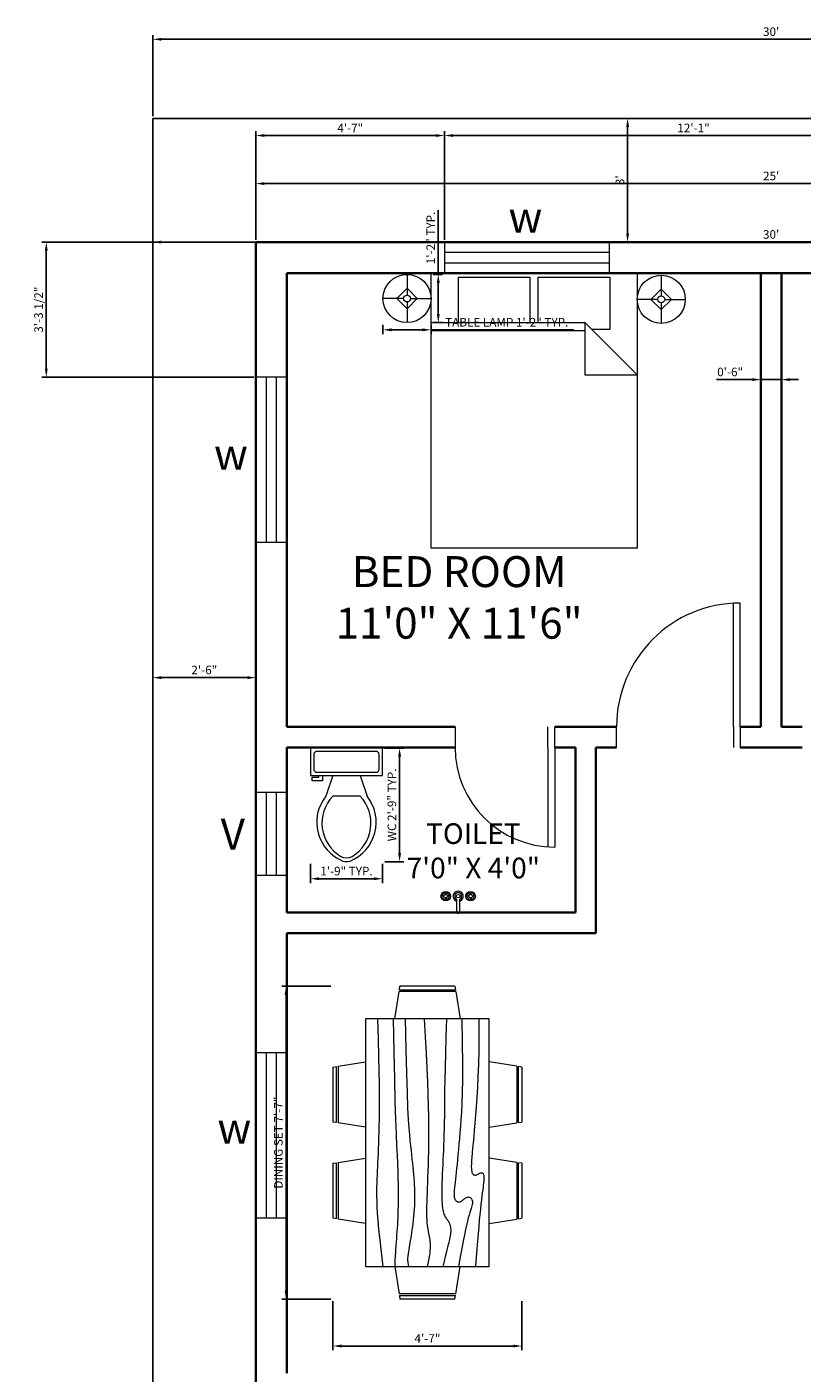
# Model space of a CAD drawing. Units: inches. Extents: x 2009 to 2890, y 2827 to 3504.
# Tile 2 of 6: x 2009 to 2235, y 3105 to 3496. Entities that reach past the tile are written whole.
import ezdxf

# ---------------------------------------------------------------- set-up
doc = ezdxf.new("R2010")
doc.units = ezdxf.units.IN
for name, color, linetype, lineweight in [('A-ANNO-DIMS', 2, 'Continuous', 18), ('A-ANNO-TEXT', 3, 'Continuous', 18), ('A-AREA-IDEN', 7, 'Continuous', 25), ('A-DOOR', 3, 'Continuous', 18), ('A-FLOR-FIXT', 9, 'Continuous', 18), ('A-FURN', 8, 'Continuous', 18), ('A-GLAZ', 4, 'Continuous', 18), ('A-WALL', 7, 'Continuous', 35), ('C-PROP', 8, 'Continuous', 25)]:
    doc.layers.add(name, color=color, linetype=linetype, lineweight=lineweight)
doc.styles.get("Standard").update_dxf_attribs({"font": 'arial.ttf'})
doc.dimstyles.new('ISO-25', dxfattribs={"dimtxt": 2.5, "dimasz": 2.5, "dimexe": 1.25, "dimexo": 0.625, "dimtad": 1, "dimdec": 0, "dimlunit": 3, "dimtxsty": 'Standard', "dimcen": 2.5, "dimadec": 0, "dimazin": 0, "dimtfac": 1, "dimtdec": 0, "dimtmove": 0, "dimatfit": 3, "dimfxl": 1, "dimarcsym": 0})

# ---------------------------------------------------------------- blocks, each defined once
blk = doc.blocks.new('Dining Set - 36 x 72 in.')
for p, q in [((-22, 27.5), (-22.1562, 26.50042)), ((-22, 27.5), (-6, 27.5)), ((-5.8437, 26.49966), (-6, 27.5)), ((6, 27.5), (5.8438, 26.50042)), ((6, 27.5), (22, 27.5)), ((22.1563, 26.49966), (22, 27.5)), ((-22.2343, 26.00059), (-23.4847, 17.99762)), ((-22.2304, 26), (-5.7608, 26)), ((-5.8416, 26.5), (-22.1534, 26.5)), ((-4.5152, 17.99762), (-5.7655, 25.99926)), ((5.7657, 26.00059), (4.5153, 17.99762)), ((5.7696, 26), (22.2392, 26)), ((22.1584, 26.5), (5.8466, 26.5)), ((23.4848, 17.99762), (22.2345, 25.99926)), ((36, 18), (-36, 18)), ((-36, 18), (-36, -18)), ((36, -18), (36, 18)), ((-45.5, 8), (-44.5004, 8.15617)), ((-45.5, 8), (-45.5, -8)), ((-44.5, -8.15843), (-44.5, 8.15338)), ((-44.0006, 8.23428), (-35.9976, 9.48474)), ((-44, 8.23041), (-44, -8.23915)), ((44.0006, 8.23428), (35.9976, 9.48474)), ((44, 8.23041), (44, -8.23915)), ((44.5, -8.15843), (44.5, 8.15338)), ((45.5, 8), (44.5005, 8.15617)), ((45.5, 8), (45.5, -8)), ((-44.4997, -8.15631), (-45.5, -8)), ((-35.9976, -9.48476), (-43.9993, -8.2345)), ((35.9976, -9.48476), (43.9993, -8.2345)), ((44.4997, -8.15631), (45.5, -8)), ((-36, -18), (36, -18)), ((-22.2343, -26.0006), (-23.4847, -17.99762)), ((-4.5152, -17.99762), (-5.7655, -25.99928)), ((5.7657, -26.0006), (4.5153, -17.99762)), ((23.4848, -17.99762), (22.2345, -25.99928)), ((-22.2304, -26), (-5.7608, -26)), ((-22, -27.5), (-22.1562, -26.50044)), ((-5.8416, -26.5), (-22.1534, -26.5)), ((-5.8437, -26.49967), (-6, -27.5)), ((5.7696, -26), (22.2392, -26)), ((6, -27.5), (5.8438, -26.50044)), ((22.1584, -26.5), (5.8466, -26.5)), ((22.1563, -26.49967), (22, -27.5)), ((-22, -27.5), (-6, -27.5)), ((6, -27.5), (22, -27.5))]:
    blk.add_line(p, q)
for points in [[(-36, 15), (-31.1772, 14.97754), (-26.8079, 14.91406), (-22.8538, 14.81543), (-19.276, 14.6875), (-16.0362, 14.53613), (-13.0957, 14.36718), (-10.4159, 14.18652), (-7.9583, 14), (-5.6904, 13.81315), (-3.6035, 13.63021), (-1.6954, 13.45508), (0.0365, 13.29166), (1.5945, 13.14388), (2.9811, 13.01562), (4.1988, 12.9108), (5.25, 12.83333), (6.1393, 12.78613), (6.8802, 12.76823), (7.4883, 12.77767), (7.9792, 12.8125), (8.3685, 12.87077), (8.6719, 12.95052), (8.9049, 13.0498), (9.0833, 13.16666), (9.2205, 13.29899), (9.3216, 13.44401), (9.3895, 13.59879), (9.4271, 13.76041), (9.4373, 13.92594), (9.4232, 14.09245), (9.3875, 14.257), (9.3333, 14.41666), (9.2638, 14.56917), (9.1836, 14.71484), (9.0975, 14.85465), (9.0104, 14.98958), (8.9272, 15.1206), (8.8529, 15.2487), (8.7922, 15.37483), (8.75, 15.5), (8.7305, 15.62467), (8.7344, 15.74739), (8.7617, 15.86621), (8.8125, 15.97916), (8.8867, 16.08431), (8.9844, 16.17968), (9.1055, 16.26334), (9.25, 16.33333), (9.4189, 16.38802), (9.6172, 16.42708), (9.8506, 16.45052), (10.125, 16.45833), (10.4463, 16.45052), (10.8203, 16.42708), (11.2529, 16.38802), (11.75, 16.33333), (12.3184, 16.26318), (12.9694, 16.17838), (13.7151, 16.07991), (14.5677, 15.96875), (15.5395, 15.84586), (16.6426, 15.71224), (17.8893, 15.56884), (19.2917, 15.41666), (20.859, 15.25667), (22.5879, 15.08984), (24.4721, 14.91715), (26.5052, 14.73958), (28.6809, 14.5581), (30.9929, 14.3737), (33.4347, 14.18733), (36, 14)], [(-36, 10), (-28.9766, 10.14274), (-23.1725, 10.20442), (-18.4241, 10.19775), (-14.5677, 10.13541), (-11.4399, 10.03011), (-8.877, 9.89453), (-6.7154, 9.74137), (-4.7917, 9.58333), (-2.9698, 9.43082), (-1.2246, 9.28515), (0.4415, 9.14534), (2.026, 9.01041), (3.5266, 8.87939), (4.9408, 8.7513), (6.266, 8.62516), (7.5, 8.5), (8.6411, 8.37549), (9.6914, 8.2539), (10.6538, 8.13818), (11.5312, 8.03125), (12.3267, 7.93603), (13.043, 7.85547), (13.6831, 7.79248), (14.25, 7.75), (14.7471, 7.7303), (15.1797, 7.73307), (15.5537, 7.75732), (15.875, 7.80208), (16.1494, 7.86637), (16.3828, 7.94922), (16.5811, 8.04964), (16.75, 8.16666), (16.8944, 8.29915), (17.0143, 8.44531), (17.1089, 8.60319), (17.1771, 8.77083), (17.218, 8.94629), (17.2305, 9.1276), (17.2137, 9.31282), (17.1667, 9.5), (17.0895, 9.6875), (16.987, 9.875), (16.8649, 10.0625), (16.7292, 10.25), (16.5856, 10.4375), (16.4401, 10.625), (16.2985, 10.8125), (16.1667, 11), (16.05, 11.18733), (15.9518, 11.3737), (15.8752, 11.5581), (15.8229, 11.73958), (15.798, 11.91715), (15.8034, 12.08984), (15.842, 12.25667), (15.9167, 12.41666), (16.0295, 12.56836), (16.1784, 12.70833), (16.3605, 12.83268), (16.5729, 12.9375), (16.8127, 13.01888), (17.0768, 13.07291), (17.3625, 13.0957), (17.6667, 13.08333), (17.9894, 13.03312), (18.3418, 12.94726), (18.7382, 12.82918), (19.1927, 12.68229), (19.7195, 12.51001), (20.3327, 12.31575), (21.0465, 12.10294), (21.875, 11.875), (22.8357, 11.63354), (23.959, 11.37304), (25.2786, 11.08618), (26.8282, 10.76562), (28.6414, 10.40405), (30.752, 9.99414), (33.1936, 9.52856), (36, 9)], [(-36, 5.5), (-30.7157, 5.3348), (-26.069, 5.20963), (-21.9946, 5.11767), (-18.4271, 5.05208), (-15.3009, 5.00602), (-12.5508, 4.97265), (-10.1112, 4.94515), (-7.9167, 4.91666), (-5.909, 4.88167), (-4.0586, 4.83984), (-2.3429, 4.79215), (-0.7396, 4.73958), (0.7739, 4.6831), (2.22, 4.6237), (3.6213, 4.56233), (5, 4.5), (6.373, 4.43782), (7.7344, 4.3776), (9.0723, 4.32129), (10.375, 4.27083), (11.6309, 4.22819), (12.8281, 4.19531), (13.9551, 4.17415), (15, 4.16666), (15.954, 4.17448), (16.819, 4.19791), (17.6001, 4.23698), (18.3021, 4.29166), (18.9299, 4.36198), (19.4883, 4.44791), (19.9823, 4.54948), (20.4167, 4.66666), (20.7969, 4.79899), (21.1302, 4.94401), (21.4245, 5.09879), (21.6875, 5.26041), (21.9271, 5.42594), (22.1511, 5.59245), (22.3672, 5.757), (22.5834, 5.91666), (22.8065, 6.06868), (23.0404, 6.21093), (23.2879, 6.34147), (23.5521, 6.45833), (23.8358, 6.55957), (24.142, 6.64323), (24.4735, 6.70735), (24.8334, 6.75), (25.2235, 6.76969), (25.642, 6.76692), (26.0858, 6.74267), (26.5521, 6.69791), (27.0379, 6.63362), (27.5404, 6.55078), (28.0565, 6.45036), (28.5834, 6.33333), (29.1242, 6.19987), (29.7071, 6.04687), (30.3661, 5.87044), (31.1354, 5.66666), (32.0493, 5.43164), (33.142, 5.16146), (34.4475, 4.85221), (36, 4.5)], [(-36, -1), (-30.7915, -0.6591), (-26.0195, -0.38216), (-21.6519, -0.16284), (-17.6563, 0.00521), (-14.0005, 0.12833), (-10.6523, 0.21289), (-7.5796, 0.26522), (-4.75, 0.29166), (-2.134, 0.29793), (0.2878, 0.28711), (2.5317, 0.26163), (4.6146, 0.22396), (6.5529, 0.17651), (8.3633, 0.12174), (10.0623, 0.06209), (11.6667, 0), (13.1899, -0.06201), (14.6341, -0.1211), (15.9982, -0.17432), (17.2813, -0.21875), (18.4823, -0.25147), (19.6003, -0.26953), (20.6343, -0.27002), (21.5834, -0.25), (22.4481, -0.20768), (23.2357, -0.14584), (23.9549, -0.06836), (24.6146, 0.02083), (25.2235, 0.11784), (25.7904, 0.21875), (26.3241, 0.31966), (26.8334, 0.41666), (27.3265, 0.50618), (27.8099, 0.58593), (28.2894, 0.65397), (28.7709, 0.70833), (29.2601, 0.74707), (29.763, 0.76823), (30.2855, 0.76985), (30.8334, 0.75), (31.4088, 0.70784), (31.9994, 0.64713), (32.589, 0.57275), (33.1615, 0.48958), (33.7008, 0.4025), (34.1908, 0.3164), (34.6153, 0.23616), (34.9584, 0.16666), (35.2099, 0.11165), (35.3848, 0.07031), (35.504, 0.04069), (35.5886, 0.02083), (35.6594, 0.00879), (35.7377, 0.0026), (35.8442, 0.00032), (36, 0)], [(-36, -6.5), (-27.1843, -6.31267), (-20.084, -6.1263), (-14.469, -5.9419), (-10.1094, -5.76042), (-6.7752, -5.58285), (-4.2363, -5.41016), (-2.2629, -5.24333), (-0.625, -5.08334), (0.8708, -4.93099), (2.2715, -4.78646), (3.5872, -4.64974), (4.8281, -4.52084), (6.0046, -4.39974), (7.127, -4.28646), (8.2053, -4.18099), (9.25, -4.08334), (10.2705, -3.99382), (11.2734, -3.91407), (12.2647, -3.84603), (13.25, -3.79167), (14.2354, -3.75293), (15.2266, -3.73177), (16.2295, -3.73015), (17.25, -3.75), (18.2912, -3.79248), (19.3451, -3.85547), (20.4009, -3.93604), (21.4479, -4.03125), (22.4754, -4.13819), (23.4727, -4.25391), (24.4289, -4.37549), (25.3334, -4.5), (26.1785, -4.62492), (26.9694, -4.74935), (27.7145, -4.87281), (28.4219, -4.99479), (29.1, -5.11483), (29.7572, -5.23242), (30.4016, -5.34709), (31.0417, -5.45834), (31.6837, -5.56437), (32.3262, -5.65821), (32.9658, -5.73153), (33.599, -5.77604), (34.2224, -5.78345), (34.8327, -5.74545), (35.4264, -5.65373), (36, -5.5)], [(-36, -10), (-26.4022, -9.81299), (-18.4675, -9.62891), (-11.9839, -9.45069), (-6.7396, -9.28125), (-2.5226, -9.12354), (0.8789, -8.98047), (3.6769, -8.85498), (6.0833, -8.75), (8.2767, -8.66765), (10.3021, -8.60677), (12.1712, -8.56543), (13.8958, -8.54167), (15.4876, -8.53353), (16.9583, -8.53907), (18.3197, -8.55632), (19.5834, -8.58334), (20.7616, -8.61841), (21.8685, -8.66081), (22.9188, -8.71004), (23.9271, -8.76563), (24.9081, -8.82707), (25.8763, -8.89388), (26.8465, -8.96558), (27.8334, -9.04167), (28.8474, -9.12118), (29.8828, -9.20117), (30.93, -9.27824), (31.9792, -9.34896), (33.0205, -9.40991), (34.0443, -9.45768), (35.0407, -9.48885), (36, -9.5)], [(-36, -14.5), (-30.0881, -14.33513), (-25.0332, -14.21224), (-20.7312, -14.12647), (-17.0781, -14.07292), (-13.97, -14.04671), (-11.3027, -14.04297), (-8.9724, -14.05681), (-6.875, -14.08334), (-4.9224, -14.11833), (-3.0905, -14.16016), (-1.3709, -14.20785), (0.2448, -14.26042), (1.7647, -14.3169), (3.1973, -14.3763), (4.5507, -14.43767), (5.8333, -14.5), (7.0554, -14.5621), (8.235, -14.62175), (9.3922, -14.67652), (10.5469, -14.72396), (11.7192, -14.76164), (12.929, -14.78711), (14.1965, -14.79794), (15.5417, -14.79167), (16.9933, -14.76424), (18.6152, -14.70508), (20.4804, -14.60197), (22.6615, -14.44271), (25.2312, -14.21509), (28.2624, -13.9069), (31.8277, -13.50594), (36, -13)]]:
    blk.add_lwpolyline(points)
blk = doc.blocks.new('Toilet - top')
for p, q in [((9.5, -6), (9.5, -2)), ((-10, -8.5), (-8, -8.5)), ((-10, -9.5), (-10, -8.5)), ((-7, -9.5), (-10, -9.5)), ((-8, -8.5), (-8, -8)), ((-7, -8), (-7, -9.5)), ((-4, -8), (-6, -14)), ((4, -8), (6, -14)), ((4, -14), (-4, -14))]:
    blk.add_line(p, q)
blk.add_lwpolyline([(10.5, -8), (10.5, 0), (-10.5, 0), (-10.5, -8)], close=True)
for points in [[(-9.5, -2), (-9.5, -6)], [(8.5, -1), (-8.5, -1)], [(-8.5, -7), (8.5, -7)]]:
    blk.add_lwpolyline(points)
for centre, radius, start, end in [((-8.62, -1.88), 0.884, 81.8699, 188.1301), ((8.62, -1.88), 0.884, 351.8699, 98.1301), ((-8.62, -6.12), 0.884, 171.8699, 278.1301), ((8.62, -6.12), 0.884, 261.8699, 8.1301), ((3.52, -21.58), 12.17, 141.4691, 247.9714), ((4.2, -21.82), 11.33, 136.3677, 238.9468), ((-3.52, -21.58), 12.17, 292.0284, 38.5307), ((-4.2, -21.82), 11.33, 301.053, 43.6321), ((0, -27.88), 4, 245.7318, 294.2682), ((0, -29), 4, 254.8605, 285.1395)]:
    blk.add_arc(centre, radius, start, end)
blk = doc.blocks.new('Bed - Queen')
for p, q in [((0, -80.00003), (0, 0)), ((0, 0), (59.99999, 0)), ((59.99999, 0), (59.99999, -80.00003)), ((7.99999, -1.2), (28.79998, -1.2)), ((7.99999, -14.4), (7.99999, -1.2)), ((28.79998, -1.2), (28.79998, -14.4)), ((31.19999, -1.2), (51.99999, -1.2)), ((31.19999, -14.4), (31.19999, -1.2)), ((51.99999, -1.2), (51.99999, -16.4)), ((0, -14.4), (44.8, -14.4)), ((59.99999, -29.6), (44.8, -14.4)), ((44.8, -14.4), (44.8, -29.6)), ((44.8, -16.8), (0, -16.8)), ((51.99999, -16.4), (46.79936, -16.4)), ((44.8, -29.6), (59.99999, -29.6)), ((59.99999, -80.00003), (0, -80.00003))]:
    blk.add_line(p, q)
blk = doc.blocks.new('Lamp - Table')
for p, q in [((0, 7), (0, 1)), ((-1, 0), (-7, 0)), ((0, 3), (-3, 0)), ((-3, 0), (0, -3)), ((3, 0), (0, 3)), ((0, -3), (3, 0)), ((1, 0), (7, 0)), ((0, -1), (0, -7))]:
    blk.add_line(p, q)
for radius in [7, 1]:
    blk.add_circle((0, 0), radius)
blk = doc.blocks.new('*D8')
at = {"layer": 'A-ANNO-DIMS', "color": 0, "lineweight": -2, "transparency": 16777216}
for p, q in [((2075.76, 3434.16), (2075.76, 3451.81)), ((2078.26, 3450.56), (2373.26, 3450.56)), ((2375.76, 3434.16), (2375.76, 3451.81))]:
    blk.add_line(p, q, dxfattribs=at)
at = {"layer": 'A-ANNO-DIMS', "color": 0, "transparency": 16777216}
for points in [[(2078.26, 3450.97), (2078.26, 3450.14), (2075.76, 3450.56)], [(2373.26, 3450.97), (2373.26, 3450.14), (2375.76, 3450.56)]]:
    blk.add_solid(points, dxfattribs=at)
at = {"layer": 'Defpoints', "color": 0, "transparency": 16777216}
for p in [(2375.76, 3450.56), (2075.76, 3433.54), (2375.76, 3433.54)]:
    blk.add_point(p, dxfattribs=at)
at = {"layer": 'A-ANNO-DIMS', "color": 0, "transparency": 16777216, "insert": (2225.76, 3452.46), "char_height": 2.5, "attachment_point": 5}
blk.add_mtext("25'", dxfattribs=at)
blk = doc.blocks.new('*D10')
at = {"layer": 'A-ANNO-DIMS', "color": 0, "lineweight": -2, "transparency": 16777216}
for p, q in [((2045.76, 3470.16), (2045.76, 3493.78)), ((2405.76, 3470.16), (2405.76, 3493.78)), ((2048.26, 3492.53), (2403.26, 3492.53))]:
    blk.add_line(p, q, dxfattribs=at)
at = {"layer": 'A-ANNO-DIMS', "color": 0, "transparency": 16777216}
for points in [[(2048.26, 3492.95), (2048.26, 3492.11), (2045.76, 3492.53)], [(2403.26, 3492.95), (2403.26, 3492.11), (2405.76, 3492.53)]]:
    blk.add_solid(points, dxfattribs=at)
at = {"layer": 'Defpoints', "color": 0, "transparency": 16777216}
for p in [(2405.76, 3492.53), (2045.76, 3469.54), (2405.76, 3469.54)]:
    blk.add_point(p, dxfattribs=at)
at = {"layer": 'A-ANNO-DIMS', "color": 0, "transparency": 16777216, "insert": (2225.76, 3494.43), "char_height": 2.5, "attachment_point": 5}
blk.add_mtext("30'", dxfattribs=at)
blk = doc.blocks.new('Faucet - Bathroom top')
for p, q in [((-4.107, 0.125), (-4.375, 0.125)), ((-3.75, 0.4788), (-3.75, 0.75)), ((-3.5, 0.482), (-3.5, 0.75)), ((-3.1461, 0.125), (-2.875, 0.125)), ((3.143, 0.125), (2.875, 0.125)), ((3.5, 0.4788), (3.5, 0.75)), ((3.75, 0.482), (3.75, 0.75)), ((4.1039, 0.125), (4.375, 0.125)), ((-4.1039, -0.125), (-4.375, -0.125)), ((-3.75, -0.4821), (-3.75, -0.75)), ((-3.5, -0.4789), (-3.5, -0.75)), ((-3.143, -0.125), (-2.875, -0.125)), ((-0.5, -0.8639), (-0.5, -4.5)), ((0.5, -4.5), (0.5, -0.8631)), ((3.1461, -0.125), (2.875, -0.125)), ((3.5, -0.4821), (3.5, -0.75)), ((3.75, -0.4789), (3.75, -0.75)), ((4.107, -0.125), (4.375, -0.125))]:
    blk.add_line(p, q)
for centre, radius in [((-3.625, 0), 1.375), ((-4.625, 0), 0.2795), ((-3.625, 0), 0.5), ((-3.625, 1), 0.2795), ((-2.625, 0), 0.2795), ((0, 0), 0.5), ((3.625, 0), 1.375), ((2.625, 0), 0.2795), ((3.625, 0), 0.5), ((3.625, 1), 0.2795), ((4.625, 0), 0.2795), ((-3.625, -1), 0.2795), ((3.625, -1), 0.2795)]:
    blk.add_circle(centre, radius)
for centre, radius, start, end in [((-3.625, 0), 1, 105.2407, 164.2093), ((-3.625, 0), 1, 16.44125, 74.07887), ((0, 0), 1.5, 289.6514, 250.3603), ((0, 0), 1, 300.3431, 239.7554), ((3.625, 0), 1, 106.12, 164.0884), ((3.625, 0), 1, 16.23422, 73.90469), ((-3.625, 0), 1, 196.2342, 253.9047), ((-3.625, 0), 1, 286.12, 344.0884), ((3.625, 0), 1, 196.4413, 254.0789), ((3.625, 0), 1, 285.2407, 344.2093), ((0, -4.5), 0.5, 180, 0)]:
    blk.add_arc(centre, radius, start, end)
blk = doc.blocks.new('*D15')
at = {"layer": 'A-ANNO-DIMS', "color": 0, "lineweight": -2, "transparency": 16777216}
for p, q in [((2184.59, 3469.54), (2185.22, 3469.54)), ((2183.97, 3436.04), (2183.97, 3467.04)), ((2184.59, 3433.54), (2185.22, 3433.54))]:
    blk.add_line(p, q, dxfattribs=at)
at = {"layer": 'A-ANNO-DIMS', "color": 0, "transparency": 16777216}
for points in [[(2183.55, 3467.04), (2184.39, 3467.04), (2183.97, 3469.54)], [(2183.55, 3436.04), (2184.39, 3436.04), (2183.97, 3433.54)]]:
    blk.add_solid(points, dxfattribs=at)
at = {"layer": 'Defpoints', "color": 0, "transparency": 16777216}
for p in [(2183.97, 3469.54), (2183.97, 3469.54), (2183.97, 3433.54)]:
    blk.add_point(p, dxfattribs=at)
at = {"layer": 'A-ANNO-DIMS', "color": 0, "transparency": 16777216, "insert": (2182.07, 3451.54), "char_height": 2.5, "attachment_point": 5, "rotation": 90}
blk.add_mtext("3'", dxfattribs=at)
blk = doc.blocks.new('*D16')
at = {"layer": 'A-ANNO-DIMS', "color": 0, "lineweight": -2, "transparency": 16777216}
for p, q in [((2045.76, 3468.91), (2045.76, 3432.29)), ((2405.76, 3468.91), (2405.76, 3432.29)), ((2403.26, 3433.54), (2048.26, 3433.54))]:
    blk.add_line(p, q, dxfattribs=at)
at = {"layer": 'A-ANNO-DIMS', "color": 0, "transparency": 16777216}
for points in [[(2048.26, 3433.96), (2048.26, 3433.12), (2045.76, 3433.54)], [(2403.26, 3433.96), (2403.26, 3433.12), (2405.76, 3433.54)]]:
    blk.add_solid(points, dxfattribs=at)
at = {"layer": 'Defpoints', "color": 0, "transparency": 16777216}
for p in [(2045.76, 3469.54), (2405.76, 3469.54), (2045.76, 3433.54)]:
    blk.add_point(p, dxfattribs=at)
at = {"layer": 'A-ANNO-DIMS', "color": 0, "transparency": 16777216, "insert": (2225.76, 3435.44), "char_height": 2.5, "attachment_point": 5}
blk.add_mtext("30'", dxfattribs=at)
blk = doc.blocks.new('*D21')
at = {"layer": 'A-ANNO-DIMS', "color": 0, "lineweight": -2, "transparency": 16777216}
for p, q in [((2045.76, 3305.32), (2045.76, 3308.09)), ((2073.26, 3306.84), (2048.26, 3306.84)), ((2075.76, 3305.32), (2075.76, 3308.09))]:
    blk.add_line(p, q, dxfattribs=at)
at = {"layer": 'A-ANNO-DIMS', "color": 0, "transparency": 16777216}
for points in [[(2048.26, 3307.25), (2048.26, 3306.42), (2045.76, 3306.84)], [(2073.26, 3307.25), (2073.26, 3306.42), (2075.76, 3306.84)]]:
    blk.add_solid(points, dxfattribs=at)
at = {"layer": 'Defpoints', "color": 0, "transparency": 16777216}
for p in [(2045.76, 3306.84), (2045.76, 3304.69), (2075.76, 3304.69)]:
    blk.add_point(p, dxfattribs=at)
at = {"layer": 'A-ANNO-DIMS', "color": 0, "transparency": 16777216, "insert": (2060.76, 3308.74), "char_height": 2.5, "attachment_point": 5}
blk.add_mtext('2\'-6"', dxfattribs=at)
blk = doc.blocks.new('WIN-48IN')
for p, q in [((0, 48), (0, 0)), ((9, 48), (0, 48)), ((3, 48), (3, 0)), ((6, 0), (6, 48)), ((9, 0), (9, 48)), ((0, 0), (9, 0))]:
    blk.add_line(p, q)
blk = doc.blocks.new('VENT-24IN')
for p, q in [((0, 24), (0, 0)), ((9, 24), (0, 24)), ((3, 24), (3, 0)), ((6, 0), (6, 24)), ((9, 0), (9, 24)), ((0, 0), (9, 0))]:
    blk.add_line(p, q)
blk = doc.blocks.new('DOOR-29IN')
for p, q in [((0, 35), (0, 29)), ((27, 29), (27, 35)), ((29, 29), (29, 35)), ((27, 29), (27, 0)), ((29, 29), (29, 0))]:
    blk.add_line(p, q)
blk.add_arc((29, 29), 29, 180, 270)
blk = doc.blocks.new('DOOR-36IN')
for p, q in [((34, 6), (34, 42)), ((36, 6), (36, 42)), ((0, 0), (0, 6)), ((34, 6), (34, 0)), ((36, 6), (36, 0))]:
    blk.add_line(p, q)
blk.add_arc((36, 6), 36, 90, 180)
blk = doc.blocks.new('*D45')
at = {"layer": 'A-ANNO-DIMS', "color": 0, "lineweight": -2, "transparency": 16777216}
for p, q in [((2112.76, 3409.49), (2112.76, 3406.77)), ((2115.26, 3408.02), (2124.26, 3408.02)), ((2126.76, 3409.49), (2126.76, 3406.77)), ((2126.76, 3408.02), (2168.33, 3408.02))]:
    blk.add_line(p, q, dxfattribs=at)
at = {"layer": 'A-ANNO-DIMS', "color": 0, "transparency": 16777216}
for points in [[(2115.26, 3408.43), (2115.26, 3407.6), (2112.76, 3408.02)], [(2124.26, 3408.43), (2124.26, 3407.6), (2126.76, 3408.02)]]:
    blk.add_solid(points, dxfattribs=at)
at = {"layer": 'Defpoints', "color": 0, "transparency": 16777216}
for p in [(2112.76, 3410.12), (2126.76, 3410.12), (2126.76, 3408.02)]:
    blk.add_point(p, dxfattribs=at)
at = {"layer": 'A-ANNO-DIMS', "color": 0, "transparency": 16777216, "insert": (2148.79, 3409.9), "char_height": 2.5, "attachment_point": 5}
blk.add_mtext('TABLE LAMP 1\'-2" TYP.', dxfattribs=at)
blk = doc.blocks.new('*D46')
at = {"layer": 'A-ANNO-DIMS', "color": 0, "lineweight": -2, "transparency": 16777216}
for p, q in [((2128.86, 3424.12), (2128.86, 3442.87)), ((2127.38, 3424.12), (2130.11, 3424.12)), ((2128.86, 3412.62), (2128.86, 3421.62)), ((2127.38, 3410.12), (2130.11, 3410.12))]:
    blk.add_line(p, q, dxfattribs=at)
at = {"layer": 'A-ANNO-DIMS', "color": 0, "transparency": 16777216}
for points in [[(2128.44, 3421.62), (2129.28, 3421.62), (2128.86, 3424.12)], [(2128.44, 3412.62), (2129.28, 3412.62), (2128.86, 3410.12)]]:
    blk.add_solid(points, dxfattribs=at)
at = {"layer": 'Defpoints', "color": 0, "transparency": 16777216}
for p in [(2126.76, 3424.12), (2128.86, 3424.12), (2126.76, 3410.12)]:
    blk.add_point(p, dxfattribs=at)
at = {"layer": 'A-ANNO-DIMS', "color": 0, "transparency": 16777216, "insert": (2126.98, 3434.74), "char_height": 2.5, "attachment_point": 5, "rotation": 90}
blk.add_mtext('1\'-2" TYP.', dxfattribs=at)
blk = doc.blocks.new('*D47')
at = {"layer": 'A-ANNO-DIMS', "color": 0, "lineweight": -2, "transparency": 16777216}
for p, q in [((2113.27, 3286.35), (2118.85, 3286.35)), ((2117.6, 3255.8), (2117.6, 3283.85)), ((2113.27, 3253.3), (2118.85, 3253.3))]:
    blk.add_line(p, q, dxfattribs=at)
at = {"layer": 'A-ANNO-DIMS', "color": 0, "transparency": 16777216}
for points in [[(2117.18, 3283.85), (2118.02, 3283.85), (2117.6, 3286.35)], [(2117.18, 3255.8), (2118.02, 3255.8), (2117.6, 3253.3)]]:
    blk.add_solid(points, dxfattribs=at)
at = {"layer": 'Defpoints', "color": 0, "transparency": 16777216}
for p in [(2112.64, 3286.35), (2117.6, 3286.35), (2112.64, 3253.3)]:
    blk.add_point(p, dxfattribs=at)
at = {"layer": 'A-ANNO-DIMS', "color": 0, "transparency": 16777216, "insert": (2115.68, 3269.82), "char_height": 2.5, "attachment_point": 5, "rotation": 90}
blk.add_mtext('WC 2\'-9" TYP.', dxfattribs=at)
blk = doc.blocks.new('*D48')
at = {"layer": 'A-ANNO-DIMS', "color": 0, "lineweight": -2, "transparency": 16777216}
for p, q in [((2091.64, 3252.67), (2091.64, 3247.09)), ((2112.64, 3252.67), (2112.64, 3247.09)), ((2094.14, 3248.34), (2110.14, 3248.34))]:
    blk.add_line(p, q, dxfattribs=at)
at = {"layer": 'A-ANNO-DIMS', "color": 0, "transparency": 16777216}
for points in [[(2094.14, 3248.76), (2094.14, 3247.93), (2091.64, 3248.34)], [(2110.14, 3248.76), (2110.14, 3247.93), (2112.64, 3248.34)]]:
    blk.add_solid(points, dxfattribs=at)
at = {"layer": 'Defpoints', "color": 0, "transparency": 16777216}
for p in [(2091.64, 3253.3), (2112.64, 3253.3), (2112.64, 3248.34)]:
    blk.add_point(p, dxfattribs=at)
at = {"layer": 'A-ANNO-DIMS', "color": 0, "transparency": 16777216, "insert": (2102.14, 3250.24), "char_height": 2.5, "attachment_point": 5}
blk.add_mtext('1\'-9" TYP.', dxfattribs=at)
blk = doc.blocks.new('*D59')
at = {"layer": 'A-ANNO-DIMS', "color": 0, "lineweight": -2, "transparency": 16777216}
for p, q in [((2097.58, 3217.06), (2083.31, 3217.06)), ((2084.56, 3214.56), (2084.56, 3128.56)), ((2097.58, 3126.06), (2083.31, 3126.06))]:
    blk.add_line(p, q, dxfattribs=at)
at = {"layer": 'A-ANNO-DIMS', "color": 0, "transparency": 16777216}
for points in [[(2084.14, 3214.56), (2084.97, 3214.56), (2084.56, 3217.06)], [(2084.14, 3128.56), (2084.97, 3128.56), (2084.56, 3126.06)]]:
    blk.add_solid(points, dxfattribs=at)
at = {"layer": 'Defpoints', "color": 0, "transparency": 16777216}
for p in [(2098.21, 3217.06), (2084.56, 3126.06), (2098.21, 3126.06)]:
    blk.add_point(p, dxfattribs=at)
at = {"layer": 'A-ANNO-DIMS', "color": 0, "transparency": 16777216, "insert": (2082.64, 3171.56), "char_height": 2.5, "attachment_point": 5, "rotation": 90}
blk.add_mtext('DINING SET 7\'-7"', dxfattribs=at)
blk = doc.blocks.new('*D60')
at = {"layer": 'A-ANNO-DIMS', "color": 0, "lineweight": -2, "transparency": 16777216}
for p, q in [((2098.21, 3125.43), (2098.21, 3111.16)), ((2153.21, 3125.43), (2153.21, 3111.16)), ((2100.71, 3112.41), (2150.71, 3112.41))]:
    blk.add_line(p, q, dxfattribs=at)
at = {"layer": 'A-ANNO-DIMS', "color": 0, "transparency": 16777216}
for points in [[(2100.71, 3112.83), (2100.71, 3111.99), (2098.21, 3112.41)], [(2150.71, 3112.83), (2150.71, 3111.99), (2153.21, 3112.41)]]:
    blk.add_solid(points, dxfattribs=at)
at = {"layer": 'Defpoints', "color": 0, "transparency": 16777216}
for p in [(2098.21, 3126.06), (2153.21, 3126.06), (2153.21, 3112.41)]:
    blk.add_point(p, dxfattribs=at)
at = {"layer": 'A-ANNO-DIMS', "color": 0, "transparency": 16777216, "insert": (2125.71, 3114.28), "char_height": 2.5, "attachment_point": 5}
blk.add_mtext('4\'-7"', dxfattribs=at)
blk = doc.blocks.new('*D76')
at = {"layer": 'A-ANNO-DIMS', "color": 0, "lineweight": -2, "transparency": 16777216}
for p, q in [((2075.76, 3434.16), (2075.76, 3465.79)), ((2130.69, 3434.16), (2130.69, 3465.79)), ((2078.26, 3464.54), (2128.19, 3464.54))]:
    blk.add_line(p, q, dxfattribs=at)
at = {"layer": 'A-ANNO-DIMS', "color": 0, "transparency": 16777216}
for points in [[(2078.26, 3464.96), (2078.26, 3464.12), (2075.76, 3464.54)], [(2128.19, 3464.96), (2128.19, 3464.12), (2130.69, 3464.54)]]:
    blk.add_solid(points, dxfattribs=at)
at = {"layer": 'Defpoints', "color": 0, "transparency": 16777216}
for p in [(2130.69, 3464.54), (2075.76, 3433.54), (2130.69, 3433.54)]:
    blk.add_point(p, dxfattribs=at)
at = {"layer": 'A-ANNO-DIMS', "color": 0, "transparency": 16777216, "insert": (2103.23, 3466.41), "char_height": 2.5, "attachment_point": 5}
blk.add_mtext('4\'-7"', dxfattribs=at)
blk = doc.blocks.new('*D77')
at = {"layer": 'A-ANNO-DIMS', "color": 0, "lineweight": -2, "transparency": 16777216}
for p, q in [((2130.69, 3434.16), (2130.69, 3465.79)), ((2275.62, 3434.16), (2275.62, 3465.79)), ((2133.19, 3464.54), (2273.12, 3464.54))]:
    blk.add_line(p, q, dxfattribs=at)
at = {"layer": 'A-ANNO-DIMS', "color": 0, "transparency": 16777216}
for points in [[(2133.19, 3464.96), (2133.19, 3464.12), (2130.69, 3464.54)], [(2273.12, 3464.96), (2273.12, 3464.12), (2275.62, 3464.54)]]:
    blk.add_solid(points, dxfattribs=at)
at = {"layer": 'Defpoints', "color": 0, "transparency": 16777216}
for p in [(2275.62, 3464.54), (2130.69, 3433.54), (2275.62, 3433.54)]:
    blk.add_point(p, dxfattribs=at)
at = {"layer": 'A-ANNO-DIMS', "color": 0, "transparency": 16777216, "insert": (2203.16, 3466.42), "char_height": 2.5, "attachment_point": 5}
blk.add_mtext('12\'-1"', dxfattribs=at)
blk = doc.blocks.new('*D79')
at = {"layer": 'A-ANNO-DIMS', "color": 0, "lineweight": -2, "transparency": 16777216}
for p, q in [((2222.76, 3423.91), (2222.76, 3392.29)), ((2228.76, 3423.91), (2228.76, 3392.29)), ((2220.26, 3393.54), (2209.87, 3393.54)), ((2228.76, 3393.54), (2222.76, 3393.54)), ((2231.26, 3393.54), (2233.76, 3393.54))]:
    blk.add_line(p, q, dxfattribs=at)
at = {"layer": 'A-ANNO-DIMS', "color": 0, "transparency": 16777216}
for points in [[(2220.26, 3393.96), (2220.26, 3393.12), (2222.76, 3393.54)], [(2231.26, 3393.96), (2231.26, 3393.12), (2228.76, 3393.54)]]:
    blk.add_solid(points, dxfattribs=at)
at = {"layer": 'Defpoints', "color": 0, "transparency": 16777216}
for p in [(2222.76, 3424.54), (2228.76, 3424.54), (2222.76, 3393.54)]:
    blk.add_point(p, dxfattribs=at)
at = {"layer": 'A-ANNO-DIMS', "color": 0, "transparency": 16777216, "insert": (2213.82, 3395.44), "char_height": 2.5, "attachment_point": 5}
blk.add_mtext('0\'-6"', dxfattribs=at)
blk = doc.blocks.new('*D81')
at = {"layer": 'A-ANNO-DIMS', "color": 0, "lineweight": -2, "transparency": 16777216}
for p, q in [((2075.14, 3433.54), (2013.51, 3433.54)), ((2014.76, 3431.04), (2014.76, 3396.72)), ((2075.14, 3394.22), (2013.51, 3394.22))]:
    blk.add_line(p, q, dxfattribs=at)
at = {"layer": 'A-ANNO-DIMS', "color": 0, "transparency": 16777216}
for points in [[(2014.35, 3431.04), (2015.18, 3431.04), (2014.76, 3433.54)], [(2014.35, 3396.72), (2015.18, 3396.72), (2014.76, 3394.22)]]:
    blk.add_solid(points, dxfattribs=at)
at = {"layer": 'Defpoints', "color": 0, "transparency": 16777216}
for p in [(2075.76, 3433.54), (2014.76, 3394.22), (2075.76, 3394.22)]:
    blk.add_point(p, dxfattribs=at)
at = {"layer": 'A-ANNO-DIMS', "color": 0, "transparency": 16777216, "insert": (2012.84, 3413.88), "char_height": 2.5, "attachment_point": 5, "rotation": 90}
blk.add_mtext('3\'-3 1/2"', dxfattribs=at)

msp = doc.modelspace()

# ---------------------------------------------------------------- linework, layer by layer
at = {"layer": 'A-WALL'}
for p, q in [((2075.76, 3433.54), (2375.76, 3433.54)), ((2075.76, 3433.54), (2075.76, 2893.54)), ((2084.76, 3424.54), (2084.76, 3292.54)), ((2084.76, 3424.54), (2228.76, 3424.54)), ((2222.76, 3424.54), (2222.76, 3292.54)), ((2228.76, 3424.54), (2228.76, 3292.54)), ((2237.76, 3424.54), (2228.76, 3424.54)), ((2084.76, 3292.54), (2133.76, 3292.54)), ((2162.76, 3292.54), (2180.76, 3292.54)), ((2222.76, 3292.54), (2216.76, 3292.54)), ((2216.76, 3292.54), (2222.76, 3292.54)), ((2228.76, 3292.54), (2234.76, 3292.54)), ((2228.76, 3292.54), (2234.76, 3292.54)), ((2084.76, 3286.54), (2133.76, 3286.54)), ((2084.76, 3286.54), (2084.76, 3238.54)), ((2168.76, 3286.54), (2162.76, 3286.54)), ((2162.76, 3286.54), (2168.76, 3286.54)), ((2168.76, 3286.54), (2168.76, 3238.54)), ((2174.76, 3286.54), (2174.76, 3238.54)), ((2174.76, 3286.54), (2180.76, 3286.54)), ((2216.76, 3286.54), (2234.76, 3286.54)), ((2084.76, 3238.54), (2168.76, 3238.54)), ((2174.76, 3238.54), (2174.76, 3232.54)), ((2084.76, 3232.54), (2174.76, 3232.54)), ((2084.76, 3232.54), (2084.76, 3104.54))]:
    msp.add_line(p, q, dxfattribs=at)
at = {"layer": 'C-PROP'}
for p, q in [((2045.76, 3433.54), (2045.76, 3469.54)), ((2075.76, 3469.54), (2045.76, 3469.54)), ((2045.76, 3469.54), (2405.76, 3469.54)), ((2405.76, 3469.54), (2045.76, 3469.54)), ((2045.76, 3469.54), (2405.76, 3469.54)), ((2405.76, 3469.54), (2045.76, 3469.54)), ((2075.76, 3469.54), (2375.76, 3469.54)), ((2045.76, 3433.54), (2045.76, 2893.54))]:
    msp.add_line(p, q, dxfattribs=at)

# ---------------------------------------------------------------- block references
at = {"layer": 'A-DOOR'}
for name, p in [('DOOR-36IN', (2180.76, 3286.54)), ('DOOR-29IN', (2133.76, 3257.54))]:
    msp.add_blockref(name, p, dxfattribs=at)
at = {"layer": 'A-FLOR-FIXT'}
for name, p in [('Toilet - top', (2102.14, 3286.35)), ('Faucet - Bathroom top', (2134.65, 3243.26))]:
    msp.add_blockref(name, p, dxfattribs=at)
at = {"layer": 'A-FURN'}
for name, p in [('Lamp - Table', (2119.76, 3417.12)), ('Bed - Queen', (2126.76, 3424.54)), ('Lamp - Table', (2193.76, 3416.89))]:
    msp.add_blockref(name, p, dxfattribs=at)
at = {"layer": 'A-FURN', "rotation": 270}
msp.add_blockref('Dining Set - 36 x 72 in.', (2125.71, 3171.56), dxfattribs=at)
at = {"layer": 'A-GLAZ', "rotation": 270.0000000000037}
msp.add_blockref('WIN-48IN', (2130.69, 3433.54), dxfattribs=at)
at = {"layer": 'A-GLAZ'}
for name, p in [('WIN-48IN', (2075.76, 3346.22)), ('VENT-24IN', (2075.76, 3249.39)), ('WIN-48IN', (2075.76, 3149.66))]:
    msp.add_blockref(name, p, dxfattribs=at)

# ---------------------------------------------------------------- texts
at = {"layer": 'A-ANNO-TEXT', "char_height": 9, "attachment_point": 1}
for s, width, insert in [('\\pxqc;w', 53.6341, (2127.41, 3445.3)), ('\\pxqc;w', 53.6341, (2041.69, 3376.36)), ('\\pxqc;V', 57.7621, (2040.17, 3265.82)), ('\\pxqc;w', 53.6341, (2042.68, 3180.31))]:
    msp.add_mtext_dynamic_manual_height_columns(s, width=width, gutter_width=12.5, heights=[0], dxfattribs=dict(at, insert=insert))
at = {"layer": 'A-AREA-IDEN', "attachment_point": 1}
for s, width, insert, char_height in [('\\pxqc;BED ROOM\\P11\'0" X 11\'6" ', 85.3364, (2092.27, 3342.18), 9), ('\\pxqc;TOILET\\P7\'0" X 4\'0"', 53.3807, (2112.38, 3264.46), 6)]:
    msp.add_mtext_dynamic_manual_height_columns(s, width=width, gutter_width=12.5, heights=[0], dxfattribs=dict(at, insert=insert, char_height=char_height))

# ---------------------------------------------------------------- dimensions: what is measured, and where the dimension line sits
at = {"layer": 'A-ANNO-DIMS'}
for base, p1, p2, override, picture, middle in [((2405.76, 3492.53), (2045.76, 3469.54), (2405.76, 3469.54), {"dimclrd": 0, "dimclre": 0, "dimclrt": 0}, '*D10', (2225.76, 3494.43)), ((2045.76, 3433.54), (2405.76, 3469.54), (2045.76, 3469.54), {"dimclrd": 0, "dimclre": 0, "dimclrt": 0}, '*D16', (2225.76, 3435.44)), ((2130.69, 3464.54), (2075.76, 3433.54), (2130.69, 3433.54), {"dimdec": 1, "dimlfac": 1, "dimrnd": 0, "dimzin": 1, "dimdsep": 46, "dimlunit": 4, "dimfrac": 2}, '*D76', (2103.23, 3466.41)), ((2275.62, 3464.54), (2130.69, 3433.54), (2275.62, 3433.54), {"dimdec": 1, "dimlfac": 1, "dimrnd": 0, "dimzin": 1, "dimdsep": 46, "dimlunit": 4, "dimfrac": 2}, '*D77', (2203.16, 3466.42)), ((2375.76, 3450.56), (2075.76, 3433.54), (2375.76, 3433.54), {"dimclrd": 0, "dimclre": 0, "dimclrt": 0}, '*D8', (2225.76, 3452.46)), ((2045.76, 3306.84), (2075.76, 3304.69), (2045.76, 3304.69), {"dimclrd": 0, "dimclre": 0, "dimclrt": 0}, '*D21', (2060.76, 3308.74)), ((2153.21, 3112.41), (2098.21, 3126.06), (2153.21, 3126.06), {"dimdec": 1, "dimlfac": 1, "dimrnd": 0, "dimzin": 1, "dimdsep": 46, "dimlunit": 4, "dimfrac": 2}, '*D60', (2125.71, 3114.28))]:
    dim = msp.add_linear_dim(base=base, p1=p1, p2=p2, dimstyle='ISO-25', override=override, dxfattribs=at)
    dim.commit()
    dim.dimension.update_dxf_attribs({"geometry": picture, "text_midpoint": middle})
for base, p1, p2, angle, override, picture, middle in [((2183.97, 3469.54), (2183.97, 3433.54), (2183.97, 3469.54), 90, {"dimclrd": 0, "dimclre": 0, "dimclrt": 0}, '*D15', (2182.07, 3451.54)), ((2014.76, 3394.22), (2075.76, 3433.54), (2075.76, 3394.22), 90, {"dimdec": 1, "dimlfac": 1, "dimrnd": 0, "dimzin": 1, "dimdsep": 46, "dimlunit": 4, "dimfrac": 2}, '*D81', (2012.84, 3413.88)), ((2222.76, 3393.54), (2228.76, 3424.54), (2222.76, 3424.54), 180, {"dimdec": 1, "dimlfac": 1, "dimrnd": 0, "dimzin": 1, "dimdsep": 46, "dimlunit": 4, "dimfrac": 2}, '*D79', (2213.82, 3395.44))]:
    dim = msp.add_linear_dim(base=base, p1=p1, p2=p2, angle=angle, dimstyle='ISO-25', override=override, dxfattribs=at)
    dim.commit()
    dim.dimension.update_dxf_attribs({"geometry": picture, "text_midpoint": middle})
for base, p1, p2, angle, text, picture, middle in [((2128.86, 3424.12), (2126.76, 3410.12), (2126.76, 3424.12), 90, '<> TYP.', '*D46', (2126.98, 3434.74)), ((2117.5987, 3286.3453), (2112.6418, 3253.2991), (2112.6418, 3286.3453), 90, 'WC <> TYP.', '*D47', (2115.6811, 3269.8222)), ((2084.56, 3126.06), (2098.21, 3217.06), (2098.21, 3126.06), 270, 'DINING SET <>', '*D59', (2082.64, 3171.56))]:
    dim = msp.add_linear_dim(base=base, p1=p1, p2=p2, angle=angle, text=text, dimstyle='ISO-25', override={"dimdec": 1, "dimlfac": 1, "dimrnd": 0, "dimzin": 1, "dimdsep": 46, "dimlunit": 4, "dimfrac": 2}, dxfattribs=at)
    dim.commit()
    dim.dimension.update_dxf_attribs({"geometry": picture, "text_midpoint": middle})
for base, p1, p2, text, picture, middle in [((2126.76, 3408.02), (2112.76, 3410.12), (2126.76, 3410.12), 'TABLE LAMP <> TYP.', '*D45', (2148.79, 3409.9)), ((2112.64, 3248.34), (2091.64, 3253.3), (2112.64, 3253.3), '<> TYP.', '*D48', (2102.14, 3250.24))]:
    dim = msp.add_linear_dim(base=base, p1=p1, p2=p2, text=text, dimstyle='ISO-25', override={"dimdec": 1, "dimlfac": 1, "dimrnd": 0, "dimzin": 1, "dimdsep": 46, "dimlunit": 4, "dimfrac": 2}, dxfattribs=at)
    dim.commit()
    dim.dimension.update_dxf_attribs({"geometry": picture, "text_midpoint": middle})

doc.saveas('drawing.dxf')
